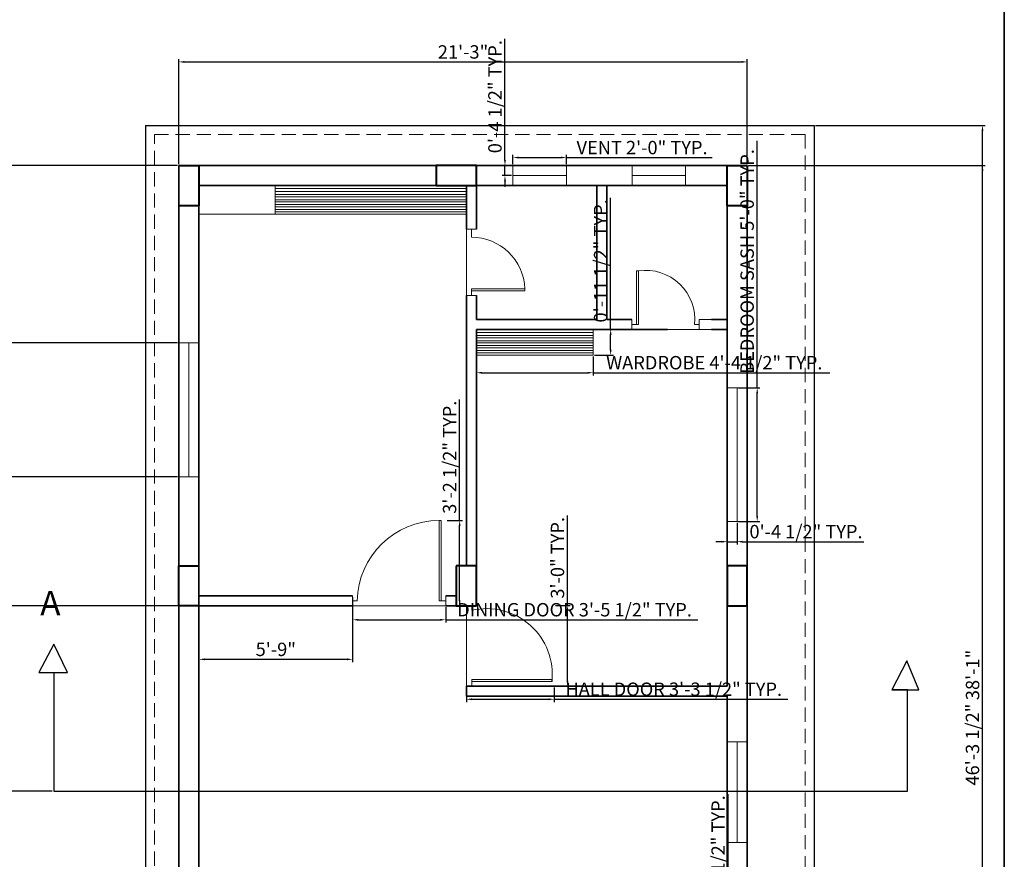
# Model space of a CAD drawing. Units: inches. Extents: x 2656 to 9931, y 1941 to 3068.
# Tile 27 of 46: x 3074 to 3515, y 2312 to 2689. Entities that reach past the tile are written whole.
import ezdxf

# ---------------------------------------------------------------- set-up
doc = ezdxf.new("R2010")
doc.units = ezdxf.units.IN
doc.linetypes.add('DASHED2', pattern=[9.525, 6.35, -3.175])
for name, color, linetype, lineweight in [('A-ANNO-DIMS', 2, 'Continuous', 18), ('A-ANNO-SYMB', 7, 'Continuous', 25), ('A-ANNO-TTLB', 7, 'Continuous', 35), ('A-COLS', 7, 'Continuous', 40), ('A-DOOR', 3, 'Continuous', 18), ('A-FLOR-CASE', 32, 'Continuous', 18), ('A-FLOR-OVHD', 252, 'DASHED2', 13), ('A-GLAZ', 4, 'Continuous', 18), ('A-WALL', 7, 'Continuous', 35), ('C-PROP', 7, 'Continuous', 25)]:
    doc.layers.add(name, color=color, linetype=linetype, lineweight=lineweight)
doc.styles.get("Standard").update_dxf_attribs({"font": 'arial.ttf'})
doc.dimstyles.new('ISO-25', dxfattribs={"dimtxt": 6, "dimasz": 2.5, "dimexe": 1.25, "dimexo": 0.625, "dimtad": 1, "dimdec": 0, "dimlunit": 3, "dimtxsty": 'Standard', "dimcen": 2.5, "dimadec": 0, "dimazin": 0, "dimtfac": 1, "dimtdec": 0, "dimtmove": 0, "dimatfit": 3, "dimfxl": 1, "dimarcsym": 0})

# ---------------------------------------------------------------- blocks, each defined once
blk = doc.blocks.new('DOOR-WC-SIDE')
for p, q in [((-0.04, 29.7), (-0.04, 0.04)), ((2.21, 29.7), (2.21, 28.12)), ((2.21, 28.12), (2.21, 26.12)), ((26.21, 3.04), (2.21, 3.04)), ((2.21, 3.04), (2.21, 2.04)), ((2.21, 0.04), (2.21, 2.04)), ((2.21, 2.04), (2.21, 2.04)), ((2.21, 2.04), (26.21, 2.04)), ((26.21, 2.04), (26.21, 3.04))]:
    blk.add_line(p, q)
blk.add_arc((2.21, 2.11), 24.02, 2.2244, 90)
blk = doc.blocks.new('DOOR-WC-FRONT')
for p, q in [((1.97, 2.25), (1.97, 26.25)), ((1.97, 26.25), (2.97, 26.25)), ((2.97, 26.25), (2.97, 2.25)), ((-0.03, 2.25), (1.97, 2.25)), ((-0.03, 0), (30.07, 0)), ((2.97, 2.25), (1.97, 2.25)), ((30.07, 2.25), (28.07, 2.25))]:
    blk.add_line(p, q)
blk.add_arc((6.14, 4.44), 22.04, 354.3038, 98.2673)
blk = doc.blocks.new('DOOR-BEDROOM-HALL')
for p, q in [((-0.04, 0), (-0.04, 36)), ((2.43, 36), (2.43, 34)), ((38.43, 3), (2.43, 3)), ((2.43, 3), (2.43, 2)), ((2.43, 0), (2.43, 2)), ((2.43, 2), (38.43, 2)), ((38.43, 2), (38.43, 3))]:
    blk.add_line(p, q)
blk.add_arc((9.01, 5.24), 29.5, 353.6889, 102.8962)
blk = doc.blocks.new('DOOR-BEDROOM-DINING')
for p, q in [((39.78, 38.25), (38.78, 38.25)), ((38.78, 38.25), (38.78, 2.25)), ((39.78, 2.25), (39.78, 38.25)), ((0.03, 2.25), (2.03, 2.25)), ((0.03, 0), (41.78, 0)), ((38.78, 2.25), (39.78, 2.25)), ((41.78, 2.25), (39.78, 2.25))]:
    blk.add_line(p, q)
blk.add_arc((38.78, 1.5), 36.75, 90, 178.8304)
blk = doc.blocks.new('WIN-60IN-SASH')
for p, q in [((4.46, 60.03), (-0.04, 60.03)), ((4.46, 0.03), (4.46, 60.03))]:
    blk.add_line(p, q)
blk = doc.blocks.new('WIN-VENT-24IN')
for p, q in [((23.99, 0), (23.99, 4.5)), ((-0.01, 0), (23.99, 0))]:
    blk.add_line(p, q)
blk = doc.blocks.new('WIN-VENT-24IN-B')
for p, q in [((24.01, 0), (24.01, 4.5)), ((0.01, 0), (0.01, 0)), ((0.01, 0), (24.01, 0))]:
    blk.add_line(p, q)
blk = doc.blocks.new('WIN-HALL')
for p, q in [((8.96, 45.14), (4.46, 45.14)), ((4.46, 45.14), (4.46, -0.02)), ((4.46, -0.02), (-0.04, -0.02))]:
    blk.add_line(p, q)
blk = doc.blocks.new('WARDROBE-LONG')
for p, q in [((34.19, 12.8), (34.19, -0.03)), ((34.19, 11.55), (119.96, 11.55)), ((34.19, 10.19), (119.96, 10.19)), ((34.19, 8.82), (119.96, 8.82)), ((34.19, 7.81), (119.96, 7.81)), ((34.19, 6.39), (119.96, 6.39)), ((34.19, 5.58), (119.96, 5.58)), ((34.19, 4.35), (119.96, 4.35)), ((34.19, 3.33), (119.96, 3.33)), ((34.19, 2.12), (119.96, 2.12)), ((34.19, 2.12), (119.96, 2.12)), ((34.19, -0.03), (34.19, 0.97)), ((34.19, 0.97), (119.96, 0.97)), ((-0.04, -0.03), (119.96, -0.03))]:
    blk.add_line(p, q)
blk = doc.blocks.new('WARDROBE-SHORT')
for p, q in [((-0.04, 10.24), (52.34, 10.24)), ((-0.04, 8.87), (52.34, 8.87)), ((52.34, 11.6), (52.34, 0.02)), ((-0.04, 7.85), (52.34, 7.85)), ((-0.04, 6.43), (52.34, 6.43)), ((-0.04, 5.63), (52.34, 5.63)), ((-0.04, 4.4), (52.34, 4.4)), ((-0.04, 3.38), (52.34, 3.38)), ((-0.04, 2.17), (52.34, 2.17)), ((-0.04, 2.17), (52.34, 2.17)), ((-0.04, 1.02), (52.34, 1.02)), ((-0.04, 0.02), (52.34, 0.02))]:
    blk.add_line(p, q)
blk = doc.blocks.new('COL-9X18')
for p, q in [((18.05, 9), (0.05, 9)), ((0.05, 9), (0.05, 0)), ((18.05, 0), (18.05, 9)), ((0.05, 0), (18.05, 0))]:
    blk.add_line(p, q)
blk = doc.blocks.new('*D27')
at = {"layer": 'A-ANNO-DIMS', "color": 0, "lineweight": -2, "transparency": 16777216}
for p, q in [((3404.55, 2523.88), (3404.55, 2634.73)), ((3396.17, 2523.88), (3405.8, 2523.88)), ((3404.55, 2466.38), (3404.55, 2521.38)), ((3396.17, 2463.88), (3405.8, 2463.88))]:
    blk.add_line(p, q, dxfattribs=at)
at = {"layer": 'A-ANNO-DIMS', "color": 0, "transparency": 16777216}
for points in [[(3404.13, 2521.38), (3404.96, 2521.38), (3404.55, 2523.88)], [(3404.13, 2466.38), (3404.96, 2466.38), (3404.55, 2463.88)]]:
    blk.add_solid(points, dxfattribs=at)
at = {"layer": 'Defpoints', "color": 0, "transparency": 16777216}
for p in [(3395.55, 2523.88), (3404.55, 2523.88), (3395.55, 2463.88)]:
    blk.add_point(p, dxfattribs=at)
at = {"layer": 'A-ANNO-DIMS', "color": 0, "transparency": 16777216, "insert": (3400.82, 2580.56), "char_height": 6, "attachment_point": 5, "rotation": 90}
blk.add_mtext('BEDROOM SASH 5\'-0" TYP.', dxfattribs=at)
blk = doc.blocks.new('*D28')
at = {"layer": 'A-ANNO-DIMS', "color": 0, "lineweight": -2, "transparency": 16777216}
for p, q in [((3391.05, 2463.26), (3391.05, 2453.63)), ((3395.55, 2463.26), (3395.55, 2453.63)), ((3388.55, 2454.88), (3386.05, 2454.88)), ((3391.05, 2454.88), (3395.55, 2454.88)), ((3398.05, 2454.88), (3452.35, 2454.88))]:
    blk.add_line(p, q, dxfattribs=at)
at = {"layer": 'A-ANNO-DIMS', "color": 0, "transparency": 16777216}
for points in [[(3388.55, 2455.3), (3388.55, 2454.46), (3391.05, 2454.88)], [(3398.05, 2455.3), (3398.05, 2454.46), (3395.55, 2454.88)]]:
    blk.add_solid(points, dxfattribs=at)
at = {"layer": 'Defpoints', "color": 0, "transparency": 16777216}
for p in [(3391.05, 2463.88), (3395.55, 2463.88), (3395.55, 2454.88)]:
    blk.add_point(p, dxfattribs=at)
at = {"layer": 'A-ANNO-DIMS', "color": 0, "transparency": 16777216, "insert": (3426.45, 2458.61), "char_height": 6, "attachment_point": 5}
blk.add_mtext('0\'-4 1/2" TYP.', dxfattribs=at)
blk = doc.blocks.new('*D37')
at = {"layer": 'A-ANNO-DIMS', "color": 0, "lineweight": -2, "transparency": 16777216}
for p, q in [((3274.05, 2389.48), (3274.05, 2382.94)), ((3313.47, 2389.48), (3313.47, 2382.94)), ((3276.55, 2384.19), (3310.97, 2384.19)), ((3313.47, 2384.19), (3418.23, 2384.19))]:
    blk.add_line(p, q, dxfattribs=at)
at = {"layer": 'A-ANNO-DIMS', "color": 0, "transparency": 16777216}
for points in [[(3276.55, 2384.6), (3276.55, 2383.77), (3274.05, 2384.19)], [(3310.97, 2384.6), (3310.97, 2383.77), (3313.47, 2384.19)]]:
    blk.add_solid(points, dxfattribs=at)
at = {"layer": 'Defpoints', "color": 0, "transparency": 16777216}
for p in [(3274.05, 2390.1), (3313.47, 2390.1), (3313.47, 2384.19)]:
    blk.add_point(p, dxfattribs=at)
at = {"layer": 'A-ANNO-DIMS', "color": 0, "transparency": 16777216, "insert": (3367.1, 2387.92), "char_height": 6, "attachment_point": 5}
blk.add_mtext('HALL DOOR 3\'-3 1/2" TYP.', dxfattribs=at)
blk = doc.blocks.new('*D38')
at = {"layer": 'A-ANNO-DIMS', "color": 0, "lineweight": -2, "transparency": 16777216}
for p, q in [((3319.39, 2426.23), (3319.39, 2466.55)), ((3314.1, 2426.23), (3320.64, 2426.23)), ((3319.39, 2392.6), (3319.39, 2423.73)), ((3314.1, 2390.1), (3320.64, 2390.1))]:
    blk.add_line(p, q, dxfattribs=at)
at = {"layer": 'A-ANNO-DIMS', "color": 0, "transparency": 16777216}
for points in [[(3318.97, 2423.73), (3319.81, 2423.73), (3319.39, 2426.23)], [(3318.97, 2392.6), (3319.81, 2392.6), (3319.39, 2390.1)]]:
    blk.add_solid(points, dxfattribs=at)
at = {"layer": 'Defpoints', "color": 0, "transparency": 16777216}
for p in [(3313.47, 2426.23), (3319.39, 2426.23), (3313.47, 2390.1)]:
    blk.add_point(p, dxfattribs=at)
at = {"layer": 'A-ANNO-DIMS', "color": 0, "transparency": 16777216, "insert": (3315.7, 2447.64), "char_height": 6, "attachment_point": 5, "rotation": 90}
blk.add_mtext('3\'-0" TYP.', dxfattribs=at)
blk = doc.blocks.new('*D39')
at = {"layer": 'A-ANNO-DIMS', "color": 0, "lineweight": -2, "transparency": 16777216}
for p, q in [((3223.02, 2425.48), (3223.02, 2418.59)), ((3264.76, 2425.48), (3264.76, 2418.59)), ((3225.52, 2419.84), (3262.26, 2419.84)), ((3264.76, 2419.84), (3377.91, 2419.84))]:
    blk.add_line(p, q, dxfattribs=at)
at = {"layer": 'A-ANNO-DIMS', "color": 0, "transparency": 16777216}
for points in [[(3225.52, 2420.26), (3225.52, 2419.42), (3223.02, 2419.84)], [(3262.26, 2420.26), (3262.26, 2419.42), (3264.76, 2419.84)]]:
    blk.add_solid(points, dxfattribs=at)
at = {"layer": 'Defpoints', "color": 0, "transparency": 16777216}
for p in [(3223.02, 2426.1), (3264.76, 2426.1), (3264.76, 2419.84)]:
    blk.add_point(p, dxfattribs=at)
at = {"layer": 'A-ANNO-DIMS', "color": 0, "transparency": 16777216, "insert": (3322.59, 2423.57), "char_height": 6, "attachment_point": 5}
blk.add_mtext('DINING DOOR 3\'-5 1/2" TYP.', dxfattribs=at)
blk = doc.blocks.new('*D40')
at = {"layer": 'A-ANNO-DIMS', "color": 0, "lineweight": -2, "transparency": 16777216}
for p, q in [((3271.03, 2464.35), (3271.03, 2518.65)), ((3265.39, 2464.35), (3272.28, 2464.35)), ((3271.03, 2428.6), (3271.03, 2461.85)), ((3265.39, 2426.1), (3272.28, 2426.1))]:
    blk.add_line(p, q, dxfattribs=at)
at = {"layer": 'A-ANNO-DIMS', "color": 0, "transparency": 16777216}
for points in [[(3270.61, 2461.85), (3271.44, 2461.85), (3271.03, 2464.35)], [(3270.61, 2428.6), (3271.44, 2428.6), (3271.03, 2426.1)]]:
    blk.add_solid(points, dxfattribs=at)
at = {"layer": 'Defpoints', "color": 0, "transparency": 16777216}
for p in [(3264.76, 2464.35), (3271.03, 2464.35), (3264.76, 2426.1)]:
    blk.add_point(p, dxfattribs=at)
at = {"layer": 'A-ANNO-DIMS', "color": 0, "transparency": 16777216, "insert": (3267.3, 2492.75), "char_height": 6, "attachment_point": 5, "rotation": 90}
blk.add_mtext('3\'-2 1/2" TYP.', dxfattribs=at)
blk = doc.blocks.new('*D42')
at = {"layer": 'A-ANNO-DIMS', "color": 0, "lineweight": -2, "transparency": 16777216}
for p, q in [((3391.52, 2287.35), (3391.52, 2341.65)), ((3384.57, 2287.35), (3392.77, 2287.35)), ((3391.52, 2251.6), (3391.52, 2284.85)), ((3384.57, 2249.1), (3392.77, 2249.1))]:
    blk.add_line(p, q, dxfattribs=at)
at = {"layer": 'A-ANNO-DIMS', "color": 0, "transparency": 16777216}
for points in [[(3391.11, 2284.85), (3391.94, 2284.85), (3391.52, 2287.35)], [(3391.11, 2251.6), (3391.94, 2251.6), (3391.52, 2249.1)]]:
    blk.add_solid(points, dxfattribs=at)
at = {"layer": 'Defpoints', "color": 0, "transparency": 16777216}
for p in [(3383.95, 2287.35), (3391.52, 2287.35), (3383.95, 2249.1)]:
    blk.add_point(p, dxfattribs=at)
at = {"layer": 'A-ANNO-DIMS', "color": 0, "transparency": 16777216, "insert": (3387.79, 2315.75), "char_height": 6, "attachment_point": 5, "rotation": 90}
blk.add_mtext('3\'-2 1/2" TYP.', dxfattribs=at)
blk = doc.blocks.new('*D43')
at = {"layer": 'A-ANNO-DIMS', "color": 0, "lineweight": -2, "transparency": 16777216}
for p, q in [((3294.97, 2624.23), (3294.97, 2628.45)), ((3297.47, 2627.2), (3316.47, 2627.2)), ((3318.97, 2624.23), (3318.97, 2628.45)), ((3318.97, 2627.2), (3384.29, 2627.2))]:
    blk.add_line(p, q, dxfattribs=at)
at = {"layer": 'A-ANNO-DIMS', "color": 0, "transparency": 16777216}
for points in [[(3297.47, 2627.62), (3297.47, 2626.78), (3294.97, 2627.2)], [(3316.47, 2627.62), (3316.47, 2626.78), (3318.97, 2627.2)]]:
    blk.add_solid(points, dxfattribs=at)
at = {"layer": 'Defpoints', "color": 0, "transparency": 16777216}
for p in [(3318.97, 2627.2), (3294.97, 2623.6), (3318.97, 2623.6)]:
    blk.add_point(p, dxfattribs=at)
at = {"layer": 'A-ANNO-DIMS', "color": 0, "transparency": 16777216, "insert": (3352.88, 2630.89), "char_height": 6, "attachment_point": 5}
blk.add_mtext('VENT 2\'-0" TYP.', dxfattribs=at)
blk = doc.blocks.new('*D44')
at = {"layer": 'A-ANNO-DIMS', "color": 0, "lineweight": -2, "transparency": 16777216}
for p, q in [((3291.37, 2626.1), (3291.37, 2680.4)), ((3294.35, 2623.6), (3290.12, 2623.6)), ((3291.37, 2619.1), (3291.37, 2623.6)), ((3294.35, 2619.1), (3290.12, 2619.1)), ((3291.37, 2616.6), (3291.37, 2614.1))]:
    blk.add_line(p, q, dxfattribs=at)
at = {"layer": 'A-ANNO-DIMS', "color": 0, "transparency": 16777216}
for points in [[(3290.96, 2626.1), (3291.79, 2626.1), (3291.37, 2623.6)], [(3290.96, 2616.6), (3291.79, 2616.6), (3291.37, 2619.1)]]:
    blk.add_solid(points, dxfattribs=at)
at = {"layer": 'Defpoints', "color": 0, "transparency": 16777216}
for p in [(3291.37, 2623.6), (3294.97, 2623.6), (3294.97, 2619.1)]:
    blk.add_point(p, dxfattribs=at)
at = {"layer": 'A-ANNO-DIMS', "color": 0, "transparency": 16777216, "insert": (3287.65, 2654.5), "char_height": 6, "attachment_point": 5, "rotation": 90}
blk.add_mtext('0\'-4 1/2" TYP.', dxfattribs=at)
blk = doc.blocks.new('*D59')
at = {"layer": 'A-ANNO-DIMS', "color": 0, "lineweight": -2, "transparency": 16777216}
for p, q in [((3278.55, 2537.89), (3278.55, 2529.41)), ((3330.93, 2537.89), (3330.93, 2529.41)), ((3281.05, 2530.66), (3328.43, 2530.66)), ((3330.93, 2530.66), (3437.17, 2530.66))]:
    blk.add_line(p, q, dxfattribs=at)
at = {"layer": 'A-ANNO-DIMS', "color": 0, "transparency": 16777216}
for points in [[(3281.05, 2531.08), (3281.05, 2530.25), (3278.55, 2530.66)], [(3328.43, 2531.08), (3328.43, 2530.25), (3330.93, 2530.66)]]:
    blk.add_solid(points, dxfattribs=at)
at = {"layer": 'Defpoints', "color": 0, "transparency": 16777216}
for p in [(3278.55, 2538.52), (3330.93, 2538.52), (3330.93, 2530.66)]:
    blk.add_point(p, dxfattribs=at)
at = {"layer": 'A-ANNO-DIMS', "color": 0, "transparency": 16777216, "insert": (3385.3, 2534.39), "char_height": 6, "attachment_point": 5}
blk.add_mtext('WARDROBE 4\'-4 1/2" TYP.', dxfattribs=at)
blk = doc.blocks.new('*D60')
at = {"layer": 'A-ANNO-DIMS', "color": 0, "lineweight": -2, "transparency": 16777216}
for p, q in [((3338.79, 2550.1), (3338.79, 2609.07)), ((3331.56, 2550.1), (3340.04, 2550.1)), ((3338.79, 2541.02), (3338.79, 2547.6)), ((3331.56, 2538.52), (3340.04, 2538.52))]:
    blk.add_line(p, q, dxfattribs=at)
at = {"layer": 'A-ANNO-DIMS', "color": 0, "transparency": 16777216}
for points in [[(3338.37, 2547.6), (3339.21, 2547.6), (3338.79, 2550.1)], [(3338.37, 2541.02), (3339.21, 2541.02), (3338.79, 2538.52)]]:
    blk.add_solid(points, dxfattribs=at)
at = {"layer": 'Defpoints', "color": 0, "transparency": 16777216}
for p in [(3330.93, 2550.1), (3338.79, 2550.1), (3330.93, 2538.52)]:
    blk.add_point(p, dxfattribs=at)
at = {"layer": 'A-ANNO-DIMS', "color": 0, "transparency": 16777216, "insert": (3335.06, 2580.83), "char_height": 6, "attachment_point": 5, "rotation": 90}
blk.add_mtext('0\'-11 1/2" TYP.', dxfattribs=at)
blk = doc.blocks.new('*D65')
at = {"layer": 'A-ANNO-DIMS', "color": 0, "lineweight": -2, "transparency": 16777216}
for p, q in [((3145.05, 2624.23), (3145.05, 2671.35)), ((3147.55, 2670.1), (3397.55, 2670.1)), ((3400.05, 2624.23), (3400.05, 2671.35))]:
    blk.add_line(p, q, dxfattribs=at)
at = {"layer": 'A-ANNO-DIMS', "color": 0, "transparency": 16777216}
for points in [[(3147.55, 2670.52), (3147.55, 2669.68), (3145.05, 2670.1)], [(3397.55, 2670.52), (3397.55, 2669.68), (3400.05, 2670.1)]]:
    blk.add_solid(points, dxfattribs=at)
at = {"layer": 'Defpoints', "color": 0, "transparency": 16777216}
for p in [(3400.05, 2670.1), (3145.05, 2623.6), (3400.05, 2623.6)]:
    blk.add_point(p, dxfattribs=at)
at = {"layer": 'A-ANNO-DIMS', "color": 0, "transparency": 16777216, "insert": (3272.55, 2673.79), "char_height": 6, "attachment_point": 5}
blk.add_mtext('21\'-3"', dxfattribs=at)
blk = doc.blocks.new('*D66')
at = {"layer": 'A-ANNO-DIMS', "color": 0, "lineweight": -2, "transparency": 16777216}
for p, q in [((3400.67, 2623.6), (3506.9, 2623.6)), ((3505.65, 2169.1), (3505.65, 2621.1)), ((3400.67, 2166.6), (3506.9, 2166.6))]:
    blk.add_line(p, q, dxfattribs=at)
at = {"layer": 'A-ANNO-DIMS', "color": 0, "transparency": 16777216}
for points in [[(3505.23, 2621.1), (3506.07, 2621.1), (3505.65, 2623.6)], [(3505.23, 2169.1), (3506.07, 2169.1), (3505.65, 2166.6)]]:
    blk.add_solid(points, dxfattribs=at)
at = {"layer": 'Defpoints', "color": 0, "transparency": 16777216}
for p in [(3400.05, 2623.6), (3505.65, 2623.6), (3400.05, 2166.6)]:
    blk.add_point(p, dxfattribs=at)
at = {"layer": 'A-ANNO-DIMS', "color": 0, "transparency": 16777216, "insert": (3501.96, 2395.1), "char_height": 6, "attachment_point": 5, "rotation": 90}
blk.add_mtext('38\'-1"', dxfattribs=at)
blk = doc.blocks.new('*D70')
at = {"layer": 'A-ANNO-DIMS', "color": 0, "lineweight": -2, "transparency": 16777216}
for p, q in [((3088.25, 2342.93), (3052.46, 2342.93)), ((3053.71, 2302.6), (3053.71, 2340.43)), ((3144.42, 2300.1), (3052.46, 2300.1))]:
    blk.add_line(p, q, dxfattribs=at)
at = {"layer": 'A-ANNO-DIMS', "color": 0, "transparency": 16777216}
for points in [[(3053.3, 2340.43), (3054.13, 2340.43), (3053.71, 2342.93)], [(3053.3, 2302.6), (3054.13, 2302.6), (3053.71, 2300.1)]]:
    blk.add_solid(points, dxfattribs=at)
at = {"layer": 'Defpoints', "color": 0, "transparency": 16777216}
for p in [(3053.71, 2342.93), (3088.87, 2342.93), (3145.05, 2300.1)]:
    blk.add_point(p, dxfattribs=at)
at = {"layer": 'A-ANNO-DIMS', "color": 0, "transparency": 16777216, "insert": (3050.02, 2321.51), "char_height": 6, "attachment_point": 5, "rotation": 90}
blk.add_mtext('3\'-7"', dxfattribs=at)
blk = doc.blocks.new('*D71')
at = {"layer": 'A-ANNO-DIMS', "color": 0, "lineweight": -2, "transparency": 16777216}
for p, q in [((3144.42, 2426.1), (3052.46, 2426.1)), ((3053.71, 2345.43), (3053.71, 2423.6)), ((3088.25, 2342.93), (3052.46, 2342.93))]:
    blk.add_line(p, q, dxfattribs=at)
at = {"layer": 'A-ANNO-DIMS', "color": 0, "transparency": 16777216}
for points in [[(3053.3, 2423.6), (3054.13, 2423.6), (3053.71, 2426.1)], [(3053.3, 2345.43), (3054.13, 2345.43), (3053.71, 2342.93)]]:
    blk.add_solid(points, dxfattribs=at)
at = {"layer": 'Defpoints', "color": 0, "transparency": 16777216}
for p in [(3053.71, 2426.1), (3145.05, 2426.1), (3088.87, 2342.93)]:
    blk.add_point(p, dxfattribs=at)
at = {"layer": 'A-ANNO-DIMS', "color": 0, "transparency": 16777216, "insert": (3050.03, 2384.51), "char_height": 6, "attachment_point": 5, "rotation": 90}
blk.add_mtext('6\'-11"', dxfattribs=at)
blk = doc.blocks.new('*D72')
at = {"layer": 'A-ANNO-DIMS', "color": 0, "lineweight": -2, "transparency": 16777216}
for p, q in [((3144.42, 2484.03), (3052.46, 2484.03)), ((3053.71, 2428.6), (3053.71, 2481.53)), ((3144.42, 2426.1), (3052.46, 2426.1))]:
    blk.add_line(p, q, dxfattribs=at)
at = {"layer": 'A-ANNO-DIMS', "color": 0, "transparency": 16777216}
for points in [[(3053.3, 2481.53), (3054.13, 2481.53), (3053.71, 2484.03)], [(3053.3, 2428.6), (3054.13, 2428.6), (3053.71, 2426.1)]]:
    blk.add_solid(points, dxfattribs=at)
at = {"layer": 'Defpoints', "color": 0, "transparency": 16777216}
for p in [(3053.71, 2484.03), (3145.05, 2484.03), (3145.05, 2426.1)]:
    blk.add_point(p, dxfattribs=at)
at = {"layer": 'A-ANNO-DIMS', "color": 0, "transparency": 16777216, "insert": (3050.03, 2455.07), "char_height": 6, "attachment_point": 5, "rotation": 90}
blk.add_mtext('4\'-10"', dxfattribs=at)
blk = doc.blocks.new('*D73')
at = {"layer": 'A-ANNO-DIMS', "color": 0, "lineweight": -2, "transparency": 16777216}
for p, q in [((3144.42, 2623.6), (3052.46, 2623.6)), ((3053.71, 2546.53), (3053.71, 2621.1)), ((3144.42, 2544.03), (3052.46, 2544.03))]:
    blk.add_line(p, q, dxfattribs=at)
at = {"layer": 'A-ANNO-DIMS', "color": 0, "transparency": 16777216}
for points in [[(3053.3, 2621.1), (3054.13, 2621.1), (3053.71, 2623.6)], [(3053.3, 2546.53), (3054.13, 2546.53), (3053.71, 2544.03)]]:
    blk.add_solid(points, dxfattribs=at)
at = {"layer": 'Defpoints', "color": 0, "transparency": 16777216}
for p in [(3053.71, 2623.6), (3145.05, 2623.6), (3145.05, 2544.03)]:
    blk.add_point(p, dxfattribs=at)
at = {"layer": 'A-ANNO-DIMS', "color": 0, "transparency": 16777216, "insert": (3049.99, 2583.82), "char_height": 6, "attachment_point": 5, "rotation": 90}
blk.add_mtext('6\'-7 1/2"', dxfattribs=at)
blk = doc.blocks.new('*D106')
at = {"layer": 'A-ANNO-DIMS', "color": 0, "lineweight": -2, "transparency": 16777216}
for p, q in [((3154.05, 2429.98), (3154.05, 2400.85)), ((3223.02, 2429.98), (3223.02, 2400.85)), ((3220.52, 2402.1), (3156.55, 2402.1))]:
    blk.add_line(p, q, dxfattribs=at)
at = {"layer": 'A-ANNO-DIMS', "color": 0, "transparency": 16777216}
for points in [[(3156.55, 2402.52), (3156.55, 2401.68), (3154.05, 2402.1)], [(3220.52, 2402.52), (3220.52, 2401.68), (3223.02, 2402.1)]]:
    blk.add_solid(points, dxfattribs=at)
at = {"layer": 'Defpoints', "color": 0, "transparency": 16777216}
for p in [(3154.05, 2430.6), (3223.02, 2430.6), (3154.05, 2402.1)]:
    blk.add_point(p, dxfattribs=at)
at = {"layer": 'A-ANNO-DIMS', "color": 0, "transparency": 16777216, "insert": (3188.53, 2405.79), "char_height": 6, "attachment_point": 5}
blk.add_mtext('5\'-9"', dxfattribs=at)
blk = doc.blocks.new('*D173')
at = {"layer": 'A-ANNO-DIMS', "color": 0, "lineweight": -2, "transparency": 16777216}
for p, q in [((3430.67, 2641.6), (3506.9, 2641.6)), ((3505.65, 2088.6), (3505.65, 2639.1)), ((3430.67, 2086.1), (3506.9, 2086.1))]:
    blk.add_line(p, q, dxfattribs=at)
at = {"layer": 'A-ANNO-DIMS', "color": 0, "transparency": 16777216}
for points in [[(3505.23, 2639.1), (3506.07, 2639.1), (3505.65, 2641.6)], [(3505.23, 2088.6), (3506.07, 2088.6), (3505.65, 2086.1)]]:
    blk.add_solid(points, dxfattribs=at)
at = {"layer": 'Defpoints', "color": 0, "transparency": 16777216}
for p in [(3430.05, 2641.6), (3505.65, 2641.6), (3430.05, 2086.1)]:
    blk.add_point(p, dxfattribs=at)
at = {"layer": 'A-ANNO-DIMS', "color": 0, "transparency": 16777216, "insert": (3501.92, 2363.85), "char_height": 6, "attachment_point": 5, "rotation": 90}
blk.add_mtext('46\'-3 1/2"', dxfattribs=at)

msp = doc.modelspace()

# ---------------------------------------------------------------- linework, layer by layer
at = {"layer": 'A-ANNO-SYMB'}
for p, q in [((3088.87, 2408.95), (3082.21, 2396.17)), ((3095.04, 2396.17), (3088.87, 2408.95)), ((3471.65, 2401.44), (3464.96, 2388.4)), ((3477.15, 2388.4), (3471.65, 2401.44)), ((3082.21, 2396.17), (3095.04, 2396.17)), ((3088.87, 2396.17), (3088.87, 2342.93)), ((3471.93, 2388.4), (3464.96, 2388.4)), ((3464.96, 2388.4), (3477.15, 2388.4)), ((3471.93, 2342.93), (3471.93, 2388.4)), ((3088.87, 2342.93), (3471.93, 2342.93))]:
    msp.add_line(p, q, dxfattribs=at)
at = {"layer": 'A-ANNO-TTLB'}
msp.add_lwpolyline([(2655.77, 3067.84), (3515.43, 3067.84), (3515.43, 1940.89), (2655.77, 1940.89)], close=True, dxfattribs=at)
at = {"layer": 'A-COLS'}
for p, q in [((3145.05, 2623.6), (3154.05, 2623.6)), ((3154.05, 2623.6), (3154.05, 2605.6)), ((3391.05, 2614.6), (3391.05, 2623.6)), ((3391.05, 2623.6), (3400.05, 2623.6)), ((3400.05, 2623.6), (3400.05, 2605.6)), ((3391.05, 2605.6), (3391.05, 2614.6)), ((3154.05, 2605.6), (3145.05, 2605.6)), ((3400.05, 2605.6), (3391.05, 2605.6)), ((3145.05, 2426.1), (3145.05, 2444.1)), ((3145.05, 2444.1), (3154.05, 2444.1)), ((3400.05, 2444.1), (3391.05, 2444.1)), ((3391.05, 2444.1), (3391.05, 2444.1)), ((3391.05, 2444.1), (3391.05, 2426.1)), ((3400.05, 2426.1), (3400.05, 2444.1)), ((3154.05, 2426.1), (3145.05, 2426.1)), ((3391.05, 2426.1), (3400.05, 2426.1))]:
    msp.add_line(p, q, dxfattribs=at)
at = {"layer": 'A-DOOR'}
for p, q in [((3274.05, 2595), (3278.55, 2595)), ((3274.05, 2565.34), (3278.55, 2565.34)), ((3348.36, 2554.6), (3348.36, 2550.1)), ((3384, 2554.6), (3378.46, 2554.6)), ((3378.46, 2554.6), (3378.46, 2550.1)), ((3378.46, 2550.1), (3384, 2550.1)), ((3223.02, 2430.6), (3223.02, 2426.1)), ((3264.76, 2430.6), (3264.76, 2426.1))]:
    msp.add_line(p, q, dxfattribs=at)
at = {"layer": 'A-FLOR-OVHD'}
for p, q in [((3134.05, 2166.6), (3134.05, 2637.6)), ((3134.05, 2637.6), (3426.05, 2637.6)), ((3426.05, 2637.6), (3426.05, 2090.1))]:
    msp.add_line(p, q, dxfattribs=at)
at = {"layer": 'A-GLAZ'}
for p, q in [((3294.97, 2623.6), (3294.97, 2614.6)), ((3318.97, 2623.6), (3318.97, 2614.6)), ((3348.4, 2623.6), (3348.4, 2614.6)), ((3372.4, 2623.6), (3372.4, 2614.6)), ((3294.97, 2614.6), (3294.97, 2619.1)), ((3348.4, 2614.6), (3348.4, 2619.1)), ((3145.05, 2544.03), (3154.05, 2544.03)), ((3391.05, 2523.88), (3400.05, 2523.88)), ((3145.05, 2484.03), (3154.05, 2484.03)), ((3154.05, 2484.03), (3149.55, 2484.03)), ((3391.05, 2463.88), (3400.05, 2463.88)), ((3400.05, 2463.88), (3395.55, 2463.88)), ((3391.05, 2365.04), (3400.05, 2365.04)), ((3391.05, 2319.88), (3400.05, 2319.88))]:
    msp.add_line(p, q, dxfattribs=at)
at = {"layer": 'A-WALL'}
for p, q in [((3145.05, 2623.6), (3145.05, 2166.6)), ((3145.05, 2623.6), (3400.05, 2623.6)), ((3400.05, 2623.6), (3400.05, 2249.1)), ((3154.05, 2614.6), (3154.05, 2166.6)), ((3154.05, 2614.6), (3391.05, 2614.6)), ((3274.05, 2614.6), (3274.05, 2595)), ((3278.55, 2614.6), (3278.55, 2595)), ((3332.55, 2614.6), (3332.55, 2554.6)), ((3337.05, 2614.6), (3337.05, 2554.6)), ((3391.05, 2614.6), (3391.05, 2390.1)), ((3274.05, 2565.34), (3274.05, 2444.1)), ((3278.55, 2565.34), (3278.55, 2554.6)), ((3278.55, 2554.6), (3332.55, 2554.6)), ((3337.05, 2554.6), (3348.36, 2554.6)), ((3384, 2554.6), (3391.05, 2554.6)), ((3278.55, 2550.1), (3278.55, 2426.1)), ((3278.55, 2550.1), (3348.36, 2550.1)), ((3278.55, 2550.1), (3364.31, 2550.1)), ((3384, 2550.1), (3391.05, 2550.1)), ((3154.05, 2430.6), (3223.02, 2430.6)), ((3264.76, 2430.6), (3269.55, 2430.6)), ((3154.05, 2426.1), (3223.02, 2426.1)), ((3264.76, 2426.1), (3278.55, 2426.1)), ((3274.05, 2390.1), (3391.05, 2390.1)), ((3274.05, 2390.1), (3274.05, 2385.6)), ((3278.55, 2385.6), (3274.05, 2385.6)), ((3278.55, 2385.6), (3391.05, 2385.6)), ((3391.05, 2385.6), (3391.05, 2253.6))]:
    msp.add_line(p, q, dxfattribs=at)
at = {"layer": 'C-PROP'}
for p, q in [((3130.05, 2641.6), (3130.05, 2086.1)), ((3130.05, 2641.6), (3430.05, 2641.6)), ((3430.05, 2641.6), (3430.05, 2086.1))]:
    msp.add_line(p, q, dxfattribs=at)

# ---------------------------------------------------------------- block references
at = {"layer": 'A-COLS'}
msp.add_blockref('COL-9X18', (3260.5, 2614.6), dxfattribs=at)
at = {"layer": 'A-COLS', "rotation": 269.9999999999977}
msp.add_blockref('COL-9X18', (3269.54, 2444.15), dxfattribs=at)
at = {"layer": 'A-DOOR'}
for name, p in [('DOOR-WC-SIDE', (3274.09, 2565.3)), ('DOOR-WC-FRONT', (3348.39, 2550.1)), ('DOOR-BEDROOM-DINING', (3222.99, 2426.1)), ('DOOR-BEDROOM-HALL', (3274.09, 2390.1))]:
    msp.add_blockref(name, p, dxfattribs=at)
at = {"layer": 'A-FLOR-CASE'}
for name, p in [('WARDROBE-LONG', (3154.09, 2601.8)), ('WARDROBE-SHORT', (3278.59, 2538.5))]:
    msp.add_blockref(name, p, dxfattribs=at)
at = {"layer": 'A-GLAZ'}
for name, p in [('WIN-VENT-24IN', (3294.99, 2619.1)), ('WIN-VENT-24IN-B', (3348.39, 2619.1)), ('WIN-60IN-SASH', (3145.09, 2484)), ('WIN-60IN-SASH', (3391.09, 2463.85)), ('WIN-HALL', (3391.09, 2319.9))]:
    msp.add_blockref(name, p, dxfattribs=at)

# ---------------------------------------------------------------- texts
at = {"layer": 'A-ANNO-SYMB', "insert": (3082.82, 2432.79), "char_height": 11, "attachment_point": 1}
msp.add_mtext_dynamic_manual_height_columns('A', width=14.9053, gutter_width=12.5, heights=[0], dxfattribs=at)

# ---------------------------------------------------------------- dimensions: what is measured, and where the dimension line sits
at = {"layer": 'A-ANNO-DIMS'}
dim = msp.add_linear_dim(base=(3400.05, 2670.1), p1=(3145.05, 2623.6), p2=(3400.05, 2623.6), dimstyle='ISO-25', override={"dimdec": 1, "dimlfac": 1, "dimrnd": 0, "dimzin": 1, "dimdsep": 46, "dimlunit": 4, "dimfrac": 2}, dxfattribs=at)
dim.commit()
dim.dimension.update_dxf_attribs({"geometry": '*D65', "text_midpoint": (3272.55, 2673.79)})
for base, p1, p2, text, picture, middle in [((3291.37, 2623.6), (3294.97, 2619.1), (3294.97, 2623.6), '<> TYP.', '*D44', (3287.65, 2654.5)), ((3404.55, 2523.88), (3395.55, 2463.88), (3395.55, 2523.88), 'BEDROOM SASH <> TYP.', '*D27', (3400.82, 2580.56)), ((3338.79, 2550.1), (3330.93, 2538.52), (3330.93, 2550.1), '<> TYP.', '*D60', (3335.06, 2580.83)), ((3271.02564883, 2464.35027301), (3264.76428, 2426.10027301), (3264.76428, 2464.35027301), '<> TYP.', '*D40', (3267.29628321, 2492.75017069)), ((3319.39, 2426.23), (3313.47, 2390.1), (3313.47, 2426.23), '<> TYP.', '*D38', (3315.7, 2447.64)), ((3391.52361648, 2287.35027301), (3383.94617811, 2249.10027301), (3383.94617811, 2287.35027301), '<> TYP.', '*D42', (3387.79425086, 2315.75017069))]:
    dim = msp.add_linear_dim(base=base, p1=p1, p2=p2, angle=90, text=text, dimstyle='ISO-25', override={"dimdec": 1, "dimlfac": 1, "dimrnd": 0, "dimzin": 1, "dimdsep": 46, "dimlunit": 4, "dimfrac": 2}, dxfattribs=at)
    dim.commit()
    dim.dimension.update_dxf_attribs({"geometry": picture, "text_midpoint": middle})
for base, p1, p2, text, picture, middle in [((3318.97, 2627.2), (3294.97, 2623.6), (3318.97, 2623.6), 'VENT <> TYP.', '*D43', (3352.88, 2630.89)), ((3330.93, 2530.66), (3278.55, 2538.52), (3330.93, 2538.52), 'WARDROBE <> TYP.', '*D59', (3385.3, 2534.39)), ((3395.55, 2454.88), (3391.05, 2463.88), (3395.55, 2463.88), '<> TYP.', '*D28', (3426.45, 2458.61)), ((3264.76, 2419.84), (3223.02, 2426.1), (3264.76, 2426.1), 'DINING DOOR <> TYP.', '*D39', (3322.59, 2423.57)), ((3313.47, 2384.19), (3274.05, 2390.1), (3313.47, 2390.1), 'HALL DOOR <> TYP.', '*D37', (3367.1, 2387.92))]:
    dim = msp.add_linear_dim(base=base, p1=p1, p2=p2, text=text, dimstyle='ISO-25', override={"dimdec": 1, "dimlfac": 1, "dimrnd": 0, "dimzin": 1, "dimdsep": 46, "dimlunit": 4, "dimfrac": 2}, dxfattribs=at)
    dim.commit()
    dim.dimension.update_dxf_attribs({"geometry": picture, "text_midpoint": middle})
for base, p1, p2, angle, picture, middle in [((3505.65, 2641.6), (3430.05, 2086.1), (3430.05, 2641.6), 90, '*D173', (3501.92, 2363.85)), ((3053.71, 2623.6), (3145.05, 2544.03), (3145.05, 2623.6), 90, '*D73', (3049.99, 2583.82)), ((3505.65, 2623.6), (3400.05, 2166.6), (3400.05, 2623.6), 90, '*D66', (3501.96, 2395.1)), ((3053.71, 2484.03), (3145.05, 2426.1), (3145.05, 2484.03), 90, '*D72', (3050.03, 2455.07)), ((3154.05, 2402.1), (3223.02, 2430.6), (3154.05, 2430.6), 180, '*D106', (3188.53, 2405.79)), ((3053.71, 2426.1), (3088.87, 2342.93), (3145.05, 2426.1), 90, '*D71', (3050.03, 2384.51)), ((3053.71, 2342.93), (3145.05, 2300.1), (3088.87, 2342.93), 90, '*D70', (3050.02, 2321.51))]:
    dim = msp.add_linear_dim(base=base, p1=p1, p2=p2, angle=angle, dimstyle='ISO-25', override={"dimdec": 1, "dimlfac": 1, "dimrnd": 0, "dimzin": 1, "dimdsep": 46, "dimlunit": 4, "dimfrac": 2}, dxfattribs=at)
    dim.commit()
    dim.dimension.update_dxf_attribs({"geometry": picture, "text_midpoint": middle})

doc.saveas('drawing.dxf')
